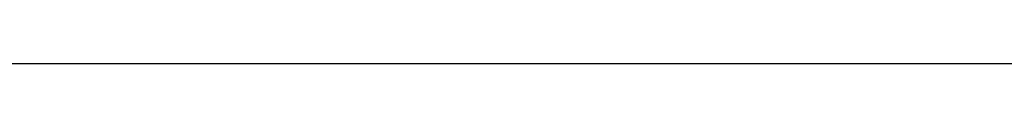
# Model space of a CAD drawing. Units: inches. Extents: x 2091 to 2899, y 967 to 2217.
# Tile 160 of 256: x 2202.5134 to 2203.1037, y 1152.2471 to 1152.2471. Entities that reach past the tile are written whole.
import ezdxf

# ---------------------------------------------------------------- set-up
doc = ezdxf.new("R2010")
doc.units = ezdxf.units.IN
doc.layers.add('A-ANNO-DIMS', color=2, linetype='Continuous', lineweight=18)
doc.styles.get("Standard").update_dxf_attribs({"font": 'arial.ttf'})
doc.dimstyles.new('ISO-25', dxfattribs={"dimtxt": 4, "dimasz": 4, "dimexe": 1.25, "dimexo": 0.625, "dimtad": 1, "dimdec": 0, "dimlunit": 3, "dimtxsty": 'Standard', "dimcen": 2.5, "dimadec": 0, "dimazin": 0, "dimtfac": 1, "dimtdec": 0, "dimtmove": 0, "dimatfit": 3, "dimfxl": 1, "dimarcsym": 0})

# ---------------------------------------------------------------- blocks, each defined once
blk = doc.blocks.new('*D91')
at = {"layer": 'A-ANNO-DIMS', "color": 0, "lineweight": -2, "transparency": 16777216}
for p, q in [((2211.65063, 1152.24706), (2098.31133, 1152.24706)), ((2099.56133, 1103.91906), (2099.56133, 1148.24706)), ((2211.5186, 1099.91906), (2098.31133, 1099.91906))]:
    blk.add_line(p, q, dxfattribs=at)
at = {"layer": 'A-ANNO-DIMS', "color": 0, "transparency": 16777216}
for points in [[(2098.89467, 1148.24706), (2100.228, 1148.24706), (2099.56133, 1152.24706)], [(2098.89467, 1103.91906), (2100.228, 1103.91906), (2099.56133, 1099.91906)]]:
    blk.add_solid(points, dxfattribs=at)
at = {"layer": 'Defpoints', "color": 0, "transparency": 16777216}
for p in [(2099.56133, 1152.24706), (2212.27563, 1152.24706), (2212.1436, 1099.91906)]:
    blk.add_point(p, dxfattribs=at)
at = {"layer": 'A-ANNO-DIMS', "color": 0, "transparency": 16777216, "insert": (2096.86812, 1126.08306), "char_height": 4, "attachment_point": 5, "rotation": 90}
blk.add_mtext('4\'-4 1/2"', dxfattribs=at)

msp = doc.modelspace()

# ---------------------------------------------------------------- dimensions: what is measured, and where the dimension line sits
at = {"layer": 'A-ANNO-DIMS'}
dim = msp.add_linear_dim(base=(2099.56133, 1152.24706), p1=(2212.1436, 1099.91906), p2=(2212.27563, 1152.24706), angle=90, dimstyle='ISO-25', override={"dimdec": 1, "dimlfac": 1, "dimrnd": 0, "dimzin": 1, "dimdsep": 46, "dimlunit": 4, "dimfrac": 2}, dxfattribs=at)
dim.commit()
dim.dimension.update_dxf_attribs({"geometry": '*D91', "text_midpoint": (2096.86812, 1126.08306)})

doc.saveas('drawing.dxf')
